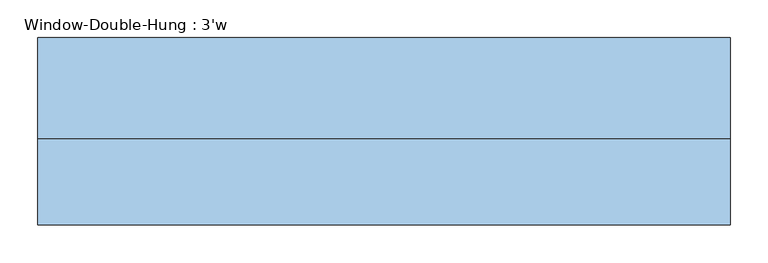
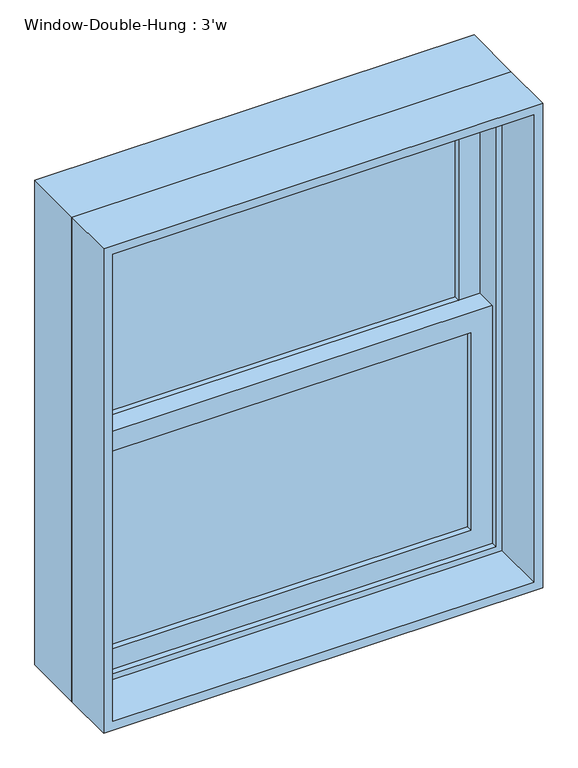
"""IFC4 building model written with IfcOpenShell, lengths in millimetres: window geometry, Window-Double-Hung : 3'w."""

from ifc_helpers import new_model, si_unit, frame, origin, place, context, project, spatial, polyline, outline, extrude, source, transform, mapped, element, save


def window_double_hung_3_w_bcdebe7f(model_context):
    return source(origin(), model_context, "Body", "SweptSolid", [
        extrude(outline(polyline([(381.0, 44.45), (381.0, 38.1), (-381.0, 38.1), (-381.0, 44.45), (381.0, 44.45)])), frame((0.0, 0.0, 990.6), z_axis=(0.0, 0.0, 1.0), x_axis=(1.0, 0.0, 0.0)), (0.0, 0.0, 1.0), 434.975),
        extrude(outline(polyline([(-381.0, 31.75), (381.0, 31.75), (381.0, 25.4), (-381.0, 25.4), (-381.0, 31.75)])), frame((0.0, 0.0, 990.6), z_axis=(0.0, 0.0, 1.0), x_axis=(1.0, 0.0, 0.0)), (0.0, 0.0, 1.0), 434.975),
        extrude(outline(polyline([(381.0, 88.9), (381.0, 82.55), (-381.0, 82.55), (-381.0, 88.9), (381.0, 88.9)])), frame((0.0, 0.0, 1470.025), z_axis=(0.0, 0.0, 1.0), x_axis=(1.0, 0.0, 0.0)), (0.0, 0.0, 1.0), 434.975),
        extrude(outline(polyline([(-381.0, 76.2), (381.0, 76.2), (381.0, 69.85), (-381.0, 69.85), (-381.0, 76.2)])), frame((0.0, 0.0, 1470.025), z_axis=(0.0, 0.0, 1.0), x_axis=(1.0, 0.0, 0.0)), (0.0, 0.0, 1.0), 434.975),
        extrude(outline(polyline([(1470.025, -425.45), (946.15, -425.45), (946.15, 425.45), (1470.025, 425.45), (1470.025, -425.45)]), holes=[polyline([(1425.575, 381.0), (990.6, 381.0), (990.6, -381.0), (1425.575, -381.0), (1425.575, 381.0)])]), frame((0.0, 12.7, 0.0), z_axis=(0.0, 1.0, 0.0), x_axis=(0.0, 0.0, 1.0)), (0.0, 0.0, 1.0), 44.45),
        extrude(outline(polyline([(1949.45, -425.45), (1425.575, -425.45), (1425.575, 425.45), (1949.45, 425.45), (1949.45, -425.45)]), holes=[polyline([(1905.0, 381.0), (1470.025, 381.0), (1470.025, -381.0), (1905.0, -381.0), (1905.0, 381.0)])]), frame((0.0, 57.15, 0.0), z_axis=(0.0, 1.0, 0.0), x_axis=(0.0, 0.0, 1.0)), (0.0, 0.0, 1.0), 44.45),
        extrude(outline(polyline([(1981.2, -457.2), (914.4, -457.2), (914.4, 457.2), (1981.2, 457.2), (1981.2, -457.2)]), holes=[polyline([(1949.45, 425.45), (946.15, 425.45), (946.15, -425.45), (1949.45, -425.45), (1949.45, 425.45)])]), frame((0.0, 0.0, 0.0), z_axis=(0.0, 1.0, 0.0), x_axis=(0.0, 0.0, 1.0)), (0.0, 0.0, 1.0), 133.35),
        extrude(outline(polyline([(1981.2, 457.2), (1981.2, -457.2), (914.4, -457.2), (914.4, 457.2), (1981.2, 457.2)]), holes=[polyline([(1962.15, 438.15), (933.45, 438.15), (933.45, -438.15), (1962.15, -438.15), (1962.15, 438.15)])]), frame((0.0, -114.3, 0.0), z_axis=(0.0, 1.0, 0.0), x_axis=(0.0, 0.0, 1.0)), (0.0, 0.0, 1.0), 114.3),
    ])


if __name__ == "__main__":
    model = new_model("IFC4")
    model_context = context("Model", 3, world=origin())
    ifc_project = project(units=[si_unit("LENGTHUNIT", "METRE", prefix="MILLI")], contexts=[model_context])
    site = spatial("IfcSite", under=ifc_project)
    building = spatial("IfcBuilding", under=site)
    placement = place(None, origin())
    window_double_hung_3_w_shape = window_double_hung_3_w_bcdebe7f(model_context)
    element("IfcWindow", 1, ObjectType="Window-Double-Hung : 3'w", at=placement, inside=building, context=model_context, shape_type="MappedRepresentation", body=[
        mapped(window_double_hung_3_w_shape, transform((0.0, 0.0, 0.0), x_axis=(1.0, 0.0, 0.0), y_axis=(0.0, 1.0, 0.0), z_axis=(0.0, 0.0, 1.0))),
    ])
    save(model, "model.ifc")

# Revit data of these elements
# Type "Window-Double-Hung : 3'w"
#   Type Mark = "23"
#   Fire Rating = "0.5h"
#   Construction Type Id = "DG-DR"
#   Assembly Code = "B2020100"
#   Analytic Construction = "Double glazing - domestic"
#   Wall Thickness [instance default] = 0' - 6"
#   Window Inset [instance default] = 0' - 0"
#   Visual Light Transmittance = 0.81
#   Thermal Resistance (R) = 1.8146 (h·ft²·°F)/BTU
#   Solar Heat Gain Coefficient = 0.76
#   Muntin Width = 2' - 6"
#   Muntin Height = 1' - 5 1/8"
#   Interior Wall Closure [instance default] = 0' - 1 1/2"
#   Rough Width = 3' - 0 1/2"
#   Rough Height = 3' - 6 1/2"
#   Frame Extension [instance default] = 0' - 1 1/4"
#   Exterior Wall Closure [instance default] = 0' - 0 1/2"
#   Extension Jamb [instance default] = 0' - 1 1/2"
#   Heat Transfer Coefficient (U) = 0.5511 BTU/(h·ft²·°F)
#   Height = 3' - 6"
#   Width = 3' - 0"
#   Top Muntin Visibility = yes
#   Indicator Visibility [instance default] = yes
#   Extension Jamb Visibility [instance default] = yes
#   Interior Trim Visibility [instance default] = yes
#   Exterior Trim Visibility [instance default] = yes
#   Define Thermal Properties by = 1
#   Bottom Muntin Visibility = yes
#   Muntin Pattern = Muntin Pattern_2x2 : Muntin Pattern_2x2
#   Interior Trim Material = Wood - Stained
#   Interior Trim = Trim-Window-Interior-Flat : Picture Frame
#   Exterior Trim Material = Clad - White
#   Exterior Trim = Trim-Window-Exterior-Flat : with Sill
#   Glass Panel Material = Glass
#   Exterior Frame Material = Clad - White
#   Interior Frame Material = Wood - Stained
#   Wall Closure = (empty or 0)
# Element 1 (IfcWindow, "Window-Double-Hung : 3'w")
#   Wall Thickness = 0' - 9"
#   Extension Jamb = 0' - 4 1/2"
#   Materials on its faces: "Wood - Stained", "Glass", "Clad - White"
# Materials
#   "Wood - Stained": class "Wood", colour RGB 224 178 126, transparency 0, Cost = 0
#   "Clad - White": class "Wood", colour RGB 242 242 238, transparency 0, Cost = 0
#   "Glass": class "Glass", colour RGB 0 128 192, transparency 0.75, Description = "Soda Lime Glass", Cost = 0
